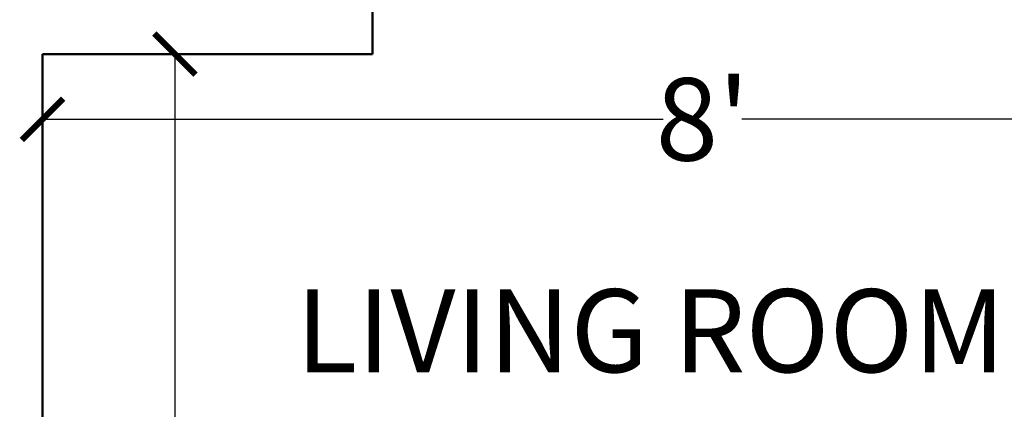
# Model space of a CAD drawing. Units: inches. Extents: x 147 to 1638, y 107 to 941.
# Tile 7 of 17: x 470 to 542, y 370 to 398. Entities that reach past the tile are written whole.
import ezdxf

# ---------------------------------------------------------------- set-up
doc = ezdxf.new("R2010")
doc.units = ezdxf.units.IN
doc.header["$MEASUREMENT"] = 0
for name, color, linetype, lineweight in [('A-ANNO-DIMS', 2, 'Continuous', 15), ('A-AREA-IDEN', 7, 'Continuous', 18), ('walls', 7, 'Continuous', 50)]:
    doc.layers.add(name, color=color, linetype=linetype, lineweight=lineweight)
doc.styles.get("Standard").update_dxf_attribs({"font": 'arial.ttf'})
doc.dimstyles.get("Standard").update_dxf_attribs({"dimtxt": 6, "dimasz": 3, "dimexe": 0.18, "dimexo": 0.0625, "dimgap": 0.09, "dimtad": 0, "dimtih": 1, "dimtoh": 1, "dimdec": 1, "dimzin": 0, "dimdsep": 46, "dimlunit": 3, "dimtxsty": 'Standard', "dimblk": 'ARCHTICK', "dimcen": 0.09, "dimadec": 0, "dimazin": 0, "dimtfac": 1, "dimtdec": 1, "dimtofl": 0, "dimtmove": 0, "dimatfit": 3, "dimfxl": 1, "dimtolj": 1, "dimtzin": 0, "dimarcsym": 0})

# ---------------------------------------------------------------- blocks, each defined once
blk = doc.blocks.new('_ArchTick')
at = {"color": 0, "linetype": 'ByBlock', "const_width": 0.15}
blk.add_lwpolyline([(-0.5, -0.5), (0.5, 0.5)], dxfattribs=at)
blk = doc.blocks.new('*D28')
at = {"layer": 'A-ANNO-DIMS', "color": 0, "lineweight": -2, "transparency": 16777216}
for p, q in [((483.882, 395.718), (481.394, 395.718)), ((481.574, 395.718), (481.574, 326.82)), ((481.574, 251.718), (481.574, 320.616)), ((483.882, 251.718), (481.394, 251.718))]:
    blk.add_line(p, q, dxfattribs=at)
at = {"layer": 'Defpoints', "color": 0, "lineweight": -2, "transparency": 16777216}
for p in [(483.944, 395.718), (481.574, 251.718), (483.944, 251.718)]:
    blk.add_point(p, dxfattribs=at)
at = {"layer": 'A-ANNO-DIMS', "color": 0, "lineweight": -2, "transparency": 16777216, "xscale": 3, "yscale": 3, "zscale": 3}
for p, rotation in [((481.574, 395.718), 90), ((481.574, 251.718), 270)]:
    blk.add_blockref('_ArchTick', p, dxfattribs=dict(at, rotation=rotation))
at = {"layer": 'A-ANNO-DIMS', "color": 0, "transparency": 16777216, "insert": (481.574, 323.718), "char_height": 6, "attachment_point": 5}
blk.add_mtext("\\A1;12'", dxfattribs=at)
blk = doc.blocks.new('*D29')
at = {"layer": 'A-ANNO-DIMS', "color": 0, "lineweight": -2, "transparency": 16777216}
for p, q in [((471.944, 391.037), (471.944, 391.154)), ((471.944, 390.974), (517.089, 390.974)), ((567.944, 390.974), (522.799, 390.974)), ((567.944, 391.037), (567.944, 391.154))]:
    blk.add_line(p, q, dxfattribs=at)
at = {"layer": 'Defpoints', "color": 0, "lineweight": -2, "transparency": 16777216}
for p in [(471.944, 390.974), (567.944, 390.974), (567.944, 390.974)]:
    blk.add_point(p, dxfattribs=at)
at = {"layer": 'A-ANNO-DIMS', "color": 0, "lineweight": -2, "transparency": 16777216, "xscale": 3, "yscale": 3, "zscale": 3, "rotation": 180}
blk.add_blockref('_ArchTick', (471.944, 390.974), dxfattribs=at)
at = {"layer": 'A-ANNO-DIMS', "color": 0, "lineweight": -2, "transparency": 16777216, "xscale": 3, "yscale": 3, "zscale": 3}
blk.add_blockref('_ArchTick', (567.944, 390.974), dxfattribs=at)
at = {"layer": 'A-ANNO-DIMS', "color": 0, "transparency": 16777216, "insert": (519.944, 390.974), "char_height": 6, "attachment_point": 5}
blk.add_mtext("\\A1;8'", dxfattribs=at)

msp = doc.modelspace()

# ---------------------------------------------------------------- linework, layer by layer
at = {"layer": 'walls'}
for p, q in [((495.944, 400.718), (495.944, 395.718)), ((471.944, 395.718), (471.944, 251.718)), ((471.944, 395.718), (495.944, 395.718))]:
    msp.add_line(p, q, dxfattribs=at)

# ---------------------------------------------------------------- texts
at = {"layer": 'A-AREA-IDEN'}
msp.add_text('LIVING ROOM 2', height=6.03059, dxfattribs=at).set_placement((490.367, 372.588))

# ---------------------------------------------------------------- dimensions: what is measured, and where the dimension line sits
at = {"layer": 'A-ANNO-DIMS'}
dim = msp.add_linear_dim(base=(481.574, 251.718), p1=(483.944, 395.718), p2=(483.944, 251.718), angle=90, dimstyle='Standard', override={"dimclrd": 0, "dimclre": 0, "dimclrt": 0}, dxfattribs=at)
dim.commit()
dim.dimension.update_dxf_attribs({"geometry": '*D28', "text_midpoint": (481.574, 323.718)})
dim = msp.add_linear_dim(base=(567.944, 390.974), p1=(471.944, 390.974), p2=(567.944, 390.974), dimstyle='Standard', override={"dimclrd": 0, "dimclre": 0, "dimclrt": 0}, dxfattribs=at)
dim.commit()
dim.dimension.update_dxf_attribs({"geometry": '*D29', "text_midpoint": (519.944, 390.974)})

doc.saveas('drawing.dxf')
